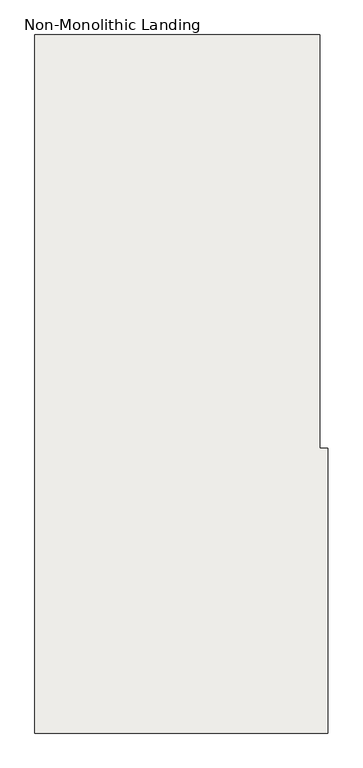
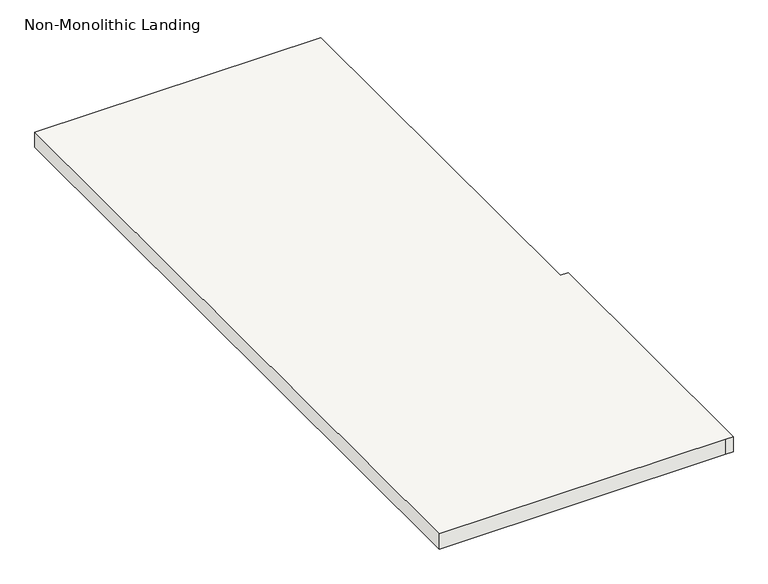
"""IFC4 building model written with IfcOpenShell, lengths in millimetres: slab geometry, Non-Monolithic Landing."""

from ifc_helpers import new_model, si_unit, origin, place, context, project, spatial, faceted_brep, source, transform, mapped, element, save


def non_monolithic_landing_a0269062(model_context):
    return source(origin(), model_context, "Body", "Brep", [
        faceted_brep([(29538.0316163, 9282.3980552, 5187.95), (29563.4316163, 9282.3980552, 5213.35), (29563.4316163, 8367.9980552, 5213.35), (29538.0316163, 8367.9980552, 5187.95), (28649.0316163, 9282.3980552, 5232.4), (28649.0316163, 7040.8480552, 5232.4), (29563.4316163, 7040.8480552, 5232.4), (29588.8316163, 7040.8480552, 5232.4), (29588.8316163, 7955.2480552, 5232.4), (29563.4316163, 7955.2480552, 5232.4), (29563.4316163, 9282.3980552, 5232.4), (29538.0316163, 8367.9980552, 5181.6), (29563.4316163, 8367.9980552, 5181.6), (29563.4316163, 7955.2480552, 5181.6), (29588.8316163, 7955.2480552, 5181.6), (29588.8316163, 7040.8480552, 5181.6), (29563.4316163, 7040.8480552, 5181.6), (28649.0316163, 7040.8480552, 5181.6), (28649.0316163, 9282.3980552, 5181.6), (29538.0316163, 9282.3980552, 5181.6)], [[[0, 1, 2, 3]], [[4, 5, 6, 7, 8, 9, 10]], [[11, 12, 13, 14, 15, 16, 17, 18, 19]], [[12, 11, 3, 2]], [[11, 19, 0, 3]], [[4, 10, 1, 0, 19, 18]], [[5, 4, 18, 17]], [[6, 5, 17, 16]], [[7, 6, 16, 15]], [[8, 7, 15, 14]], [[9, 8, 14, 13]], [[10, 9, 13, 12, 2, 1]]]),
    ])


if __name__ == "__main__":
    model = new_model("IFC4")
    model_context = context("Model", 3, world=origin())
    ifc_project = project(units=[si_unit("LENGTHUNIT", "METRE", prefix="MILLI")], contexts=[model_context])
    site = spatial("IfcSite", under=ifc_project)
    building = spatial("IfcBuilding", under=site)
    placement = place(None, origin())
    non_monolithic_landing_shape = non_monolithic_landing_a0269062(model_context)
    element("IfcSlab", 1, ObjectType="Non-Monolithic Landing", at=placement, inside=building, context=model_context, shape_type="MappedRepresentation", body=[
        mapped(non_monolithic_landing_shape, transform((0.0, 0.0, 0.0), x_axis=(1.0, 0.0, 0.0), y_axis=(0.0, 1.0, 0.0), z_axis=(0.0, 0.0, 1.0))),
    ])
    save(model, "model.ifc")
